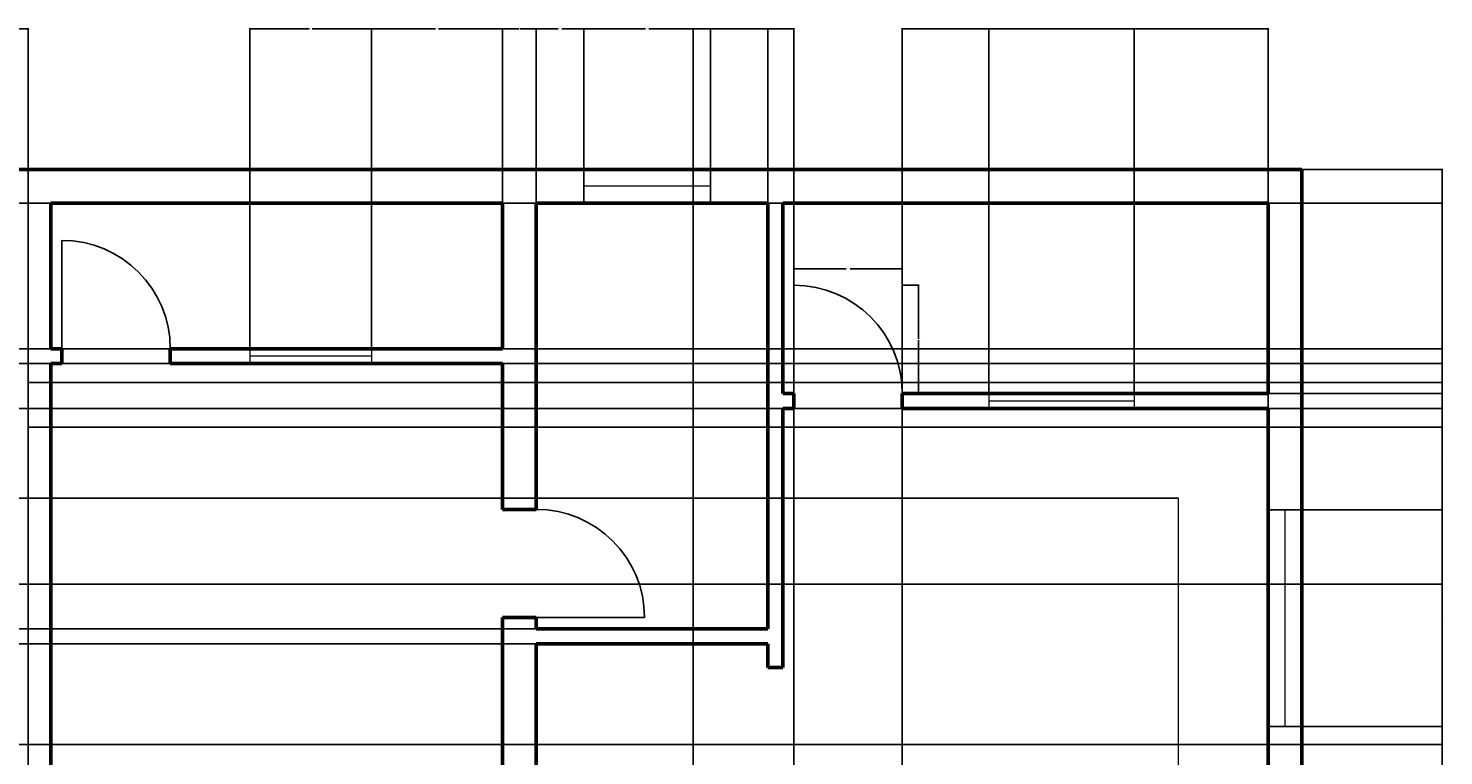
# Model space of a CAD drawing. Units: inches. Extents: x 2479 to 3284, y 2154 to 2936.
# Tile 8 of 8: x 2905 to 3284, y 2741 to 2936. Entities that reach past the tile are written whole.
import ezdxf

# ---------------------------------------------------------------- set-up
doc = ezdxf.new("R2010")
doc.units = ezdxf.units.IN
for name, color, linetype, lineweight in [('A-ANNO-DIMS', 2, 'Continuous', 18), ('A-DOOR', 3, 'Continuous', 25), ('A-FLOR-CASE', 8, 'Continuous', 18), ('A-GLAZ', 4, 'Continuous', 18), ('A-WALL', 7, 'Continuous', 50)]:
    doc.layers.add(name, color=color, linetype=linetype, lineweight=lineweight)
doc.styles.get("Standard").update_dxf_attribs({"font": 'arial.ttf'})
doc.dimstyles.get("Standard").update_dxf_attribs({"dimtxt": 0.18, "dimasz": 0.18, "dimexe": 0.18, "dimexo": 0.0625, "dimgap": 0.09, "dimtad": 0, "dimtih": 1, "dimtoh": 1, "dimdec": 4, "dimzin": 0, "dimdsep": 46, "dimtxsty": 'Standard', "dimcen": 0.09, "dimadec": 0, "dimazin": 0, "dimtfac": 1, "dimtdec": 4, "dimtofl": 0, "dimtmove": 0, "dimatfit": 3, "dimfxl": 1, "dimtolj": 1, "dimtzin": 0, "dimarcsym": 0})

# ---------------------------------------------------------------- blocks, each defined once
blk = doc.blocks.new('DOOR-SWING-29IN')
blk.add_line((29, 0), (0, 0))
blk.add_arc((29, 0), 29, 90, 180)
blk = doc.blocks.new('*D3')
at = {"layer": 'A-ANNO-DIMS', "color": 0, "lineweight": -2, "transparency": 16777216}
for p, q in [((3139.27, 2866.74), (3143.74, 2866.74)), ((3143.56, 2866.56), (3143.56, 2852.42)), ((3143.56, 2837.92), (3143.56, 2852.06)), ((3139.27, 2837.74), (3143.74, 2837.74))]:
    blk.add_line(p, q, dxfattribs=at)
at = {"layer": 'A-ANNO-DIMS', "color": 0, "transparency": 16777216}
for points in [[(3143.53, 2866.56), (3143.59, 2866.56), (3143.56, 2866.74)], [(3143.53, 2837.92), (3143.59, 2837.92), (3143.56, 2837.74)]]:
    blk.add_solid(points, dxfattribs=at)
at = {"layer": 'Defpoints', "color": 0, "transparency": 16777216}
for p in [(3139.21, 2866.74), (3139.21, 2837.74), (3143.56, 2837.74)]:
    blk.add_point(p, dxfattribs=at)
at = {"layer": 'A-ANNO-DIMS', "color": 0, "transparency": 16777216, "insert": (3143.56, 2852.24), "char_height": 0.18, "attachment_point": 5}
blk.add_mtext('\\A1;DOOR 29 TYP.', dxfattribs=at)
blk = doc.blocks.new('*D4')
at = {"layer": 'A-ANNO-DIMS', "color": 0, "lineweight": -2, "transparency": 16777216}
for p, q in [((3110.21, 2866.8), (3110.21, 2871.27)), ((3110.39, 2871.09), (3124.18, 2871.09)), ((3139.03, 2871.09), (3125.24, 2871.09)), ((3139.21, 2866.8), (3139.21, 2871.27))]:
    blk.add_line(p, q, dxfattribs=at)
at = {"layer": 'A-ANNO-DIMS', "color": 0, "transparency": 16777216}
for points in [[(3110.39, 2871.12), (3110.39, 2871.06), (3110.21, 2871.09)], [(3139.03, 2871.12), (3139.03, 2871.06), (3139.21, 2871.09)]]:
    blk.add_solid(points, dxfattribs=at)
at = {"layer": 'Defpoints', "color": 0, "transparency": 16777216}
for p in [(3139.21, 2871.09), (3110.21, 2866.74), (3139.21, 2866.74)]:
    blk.add_point(p, dxfattribs=at)
at = {"layer": 'A-ANNO-DIMS', "color": 0, "transparency": 16777216, "insert": (3124.71, 2871.09), "char_height": 0.18, "attachment_point": 5}
blk.add_mtext('\\A1;29 TYP.', dxfattribs=at)
blk = doc.blocks.new('*D9')
at = {"layer": 'A-ANNO-DIMS', "color": 0, "lineweight": -2, "transparency": 16777216}
for p, q in [((2517.21, 2897.8), (2517.21, 2935.52)), ((2517.39, 2935.34), (2710.92, 2935.34)), ((2905.03, 2935.34), (2711.5, 2935.34)), ((2905.21, 2888.8), (2905.21, 2935.52))]:
    blk.add_line(p, q, dxfattribs=at)
at = {"layer": 'A-ANNO-DIMS', "color": 0, "transparency": 16777216}
for points in [[(2517.39, 2935.37), (2517.39, 2935.31), (2517.21, 2935.34)], [(2905.03, 2935.37), (2905.03, 2935.31), (2905.21, 2935.34)]]:
    blk.add_solid(points, dxfattribs=at)
at = {"layer": 'Defpoints', "color": 0, "transparency": 16777216}
for p in [(2905.21, 2935.34), (2517.21, 2897.74), (2905.21, 2888.74)]:
    blk.add_point(p, dxfattribs=at)
at = {"layer": 'A-ANNO-DIMS', "color": 0, "transparency": 16777216, "insert": (2711.21, 2935.34), "char_height": 0.18, "attachment_point": 5}
blk.add_mtext('\\A1;388', dxfattribs=at)
blk = doc.blocks.new('*D10')
at = {"layer": 'A-ANNO-DIMS', "color": 0, "lineweight": -2, "transparency": 16777216}
for p, q in [((3246.27, 2897.74), (3283.99, 2897.74)), ((3283.81, 2897.56), (3283.81, 2715.92)), ((3283.81, 2533.92), (3283.81, 2715.56)), ((3237.27, 2533.74), (3283.99, 2533.74))]:
    blk.add_line(p, q, dxfattribs=at)
at = {"layer": 'A-ANNO-DIMS', "color": 0, "transparency": 16777216}
for points in [[(3283.78, 2897.56), (3283.84, 2897.56), (3283.81, 2897.74)], [(3283.78, 2533.92), (3283.84, 2533.92), (3283.81, 2533.74)]]:
    blk.add_solid(points, dxfattribs=at)
at = {"layer": 'Defpoints', "color": 0, "transparency": 16777216}
for p in [(3246.21, 2897.74), (3283.81, 2897.74), (3237.21, 2533.74)]:
    blk.add_point(p, dxfattribs=at)
at = {"layer": 'A-ANNO-DIMS', "color": 0, "transparency": 16777216, "insert": (3283.81, 2715.74), "char_height": 0.18, "attachment_point": 5}
blk.add_mtext('\\A1;364', dxfattribs=at)
blk = doc.blocks.new('*D11')
at = {"layer": 'A-ANNO-DIMS', "color": 0, "lineweight": -2, "transparency": 16777216}
for p, q in [((2845.21, 2542.8), (2845.21, 2935.52)), ((2845.39, 2935.34), (2874.99, 2935.34)), ((2905.03, 2935.34), (2875.43, 2935.34)), ((2905.21, 2542.8), (2905.21, 2935.52))]:
    blk.add_line(p, q, dxfattribs=at)
at = {"layer": 'A-ANNO-DIMS', "color": 0, "transparency": 16777216}
for points in [[(2845.39, 2935.37), (2845.39, 2935.31), (2845.21, 2935.34)], [(2905.03, 2935.37), (2905.03, 2935.31), (2905.21, 2935.34)]]:
    blk.add_solid(points, dxfattribs=at)
at = {"layer": 'Defpoints', "color": 0, "transparency": 16777216}
for p in [(2905.21, 2935.34), (2845.21, 2542.74), (2905.21, 2542.74)]:
    blk.add_point(p, dxfattribs=at)
at = {"layer": 'A-ANNO-DIMS', "color": 0, "transparency": 16777216, "insert": (2875.21, 2935.34), "char_height": 0.18, "attachment_point": 5}
blk.add_mtext('\\A1;60', dxfattribs=at)
blk = doc.blocks.new('*D32')
at = {"layer": 'A-ANNO-DIMS', "color": 0, "lineweight": -2, "transparency": 16777216}
for p, q in [((2905.27, 2840.74), (3283.99, 2840.74)), ((3283.81, 2840.56), (3283.81, 2834.92)), ((3283.81, 2828.92), (3283.81, 2834.56)), ((2905.27, 2828.74), (3283.99, 2828.74))]:
    blk.add_line(p, q, dxfattribs=at)
at = {"layer": 'A-ANNO-DIMS', "color": 0, "transparency": 16777216}
for points in [[(3283.78, 2840.56), (3283.84, 2840.56), (3283.81, 2840.74)], [(3283.78, 2828.92), (3283.84, 2828.92), (3283.81, 2828.74)]]:
    blk.add_solid(points, dxfattribs=at)
at = {"layer": 'Defpoints', "color": 0, "transparency": 16777216}
for p in [(2905.21, 2840.74), (3283.81, 2840.74), (2905.21, 2828.74)]:
    blk.add_point(p, dxfattribs=at)
at = {"layer": 'A-ANNO-DIMS', "color": 0, "transparency": 16777216, "insert": (3283.81, 2834.74), "char_height": 0.18, "attachment_point": 5}
blk.add_mtext('\\A1;12', dxfattribs=at)
blk = doc.blocks.new('*D34')
at = {"layer": 'A-ANNO-DIMS', "color": 0, "lineweight": -2, "transparency": 16777216}
for p, q in [((2856.82, 2897.74), (3283.99, 2897.74)), ((3283.81, 2897.56), (3283.81, 2893.42)), ((3283.81, 2888.92), (3283.81, 2893.06)), ((2856.82, 2888.74), (3283.99, 2888.74))]:
    blk.add_line(p, q, dxfattribs=at)
at = {"layer": 'A-ANNO-DIMS', "color": 0, "transparency": 16777216}
for points in [[(3283.78, 2897.56), (3283.84, 2897.56), (3283.81, 2897.74)], [(3283.78, 2888.92), (3283.84, 2888.92), (3283.81, 2888.74)]]:
    blk.add_solid(points, dxfattribs=at)
at = {"layer": 'Defpoints', "color": 0, "transparency": 16777216}
for p in [(2856.76, 2897.74), (3283.81, 2897.74), (2856.76, 2888.74)]:
    blk.add_point(p, dxfattribs=at)
at = {"layer": 'A-ANNO-DIMS', "color": 0, "transparency": 16777216, "insert": (3283.81, 2893.24), "char_height": 0.18, "attachment_point": 5}
blk.add_mtext('\\A1;9', dxfattribs=at)
blk = doc.blocks.new('*D58')
at = {"layer": 'A-ANNO-DIMS', "color": 0, "lineweight": -2, "transparency": 16777216}
for p, q in [((2718.27, 2888.74), (3283.99, 2888.74)), ((3283.81, 2888.56), (3283.81, 2869.42)), ((3283.81, 2849.92), (3283.81, 2869.06)), ((2718.27, 2849.74), (3283.99, 2849.74))]:
    blk.add_line(p, q, dxfattribs=at)
at = {"layer": 'A-ANNO-DIMS', "color": 0, "transparency": 16777216}
for points in [[(3283.78, 2888.56), (3283.84, 2888.56), (3283.81, 2888.74)], [(3283.78, 2849.92), (3283.84, 2849.92), (3283.81, 2849.74)]]:
    blk.add_solid(points, dxfattribs=at)
at = {"layer": 'Defpoints', "color": 0, "transparency": 16777216}
for p in [(2718.21, 2888.74), (3283.81, 2888.74), (2718.21, 2849.74)]:
    blk.add_point(p, dxfattribs=at)
at = {"layer": 'A-ANNO-DIMS', "color": 0, "transparency": 16777216, "insert": (3283.81, 2869.24), "char_height": 0.18, "attachment_point": 5}
blk.add_mtext('\\A1;39', dxfattribs=at)
blk = doc.blocks.new('*D59')
at = {"layer": 'A-ANNO-DIMS', "color": 0, "lineweight": -2, "transparency": 16777216}
for p, q in [((2839.27, 2845.74), (3283.99, 2845.74)), ((3283.81, 2845.56), (3283.81, 2816.42)), ((3283.81, 2786.92), (3283.81, 2816.06)), ((2712.27, 2786.74), (3283.99, 2786.74))]:
    blk.add_line(p, q, dxfattribs=at)
at = {"layer": 'A-ANNO-DIMS', "color": 0, "transparency": 16777216}
for points in [[(3283.78, 2845.56), (3283.84, 2845.56), (3283.81, 2845.74)], [(3283.78, 2786.92), (3283.84, 2786.92), (3283.81, 2786.74)]]:
    blk.add_solid(points, dxfattribs=at)
at = {"layer": 'Defpoints', "color": 0, "transparency": 16777216}
for p in [(2839.21, 2845.74), (3283.81, 2845.74), (2712.21, 2786.74)]:
    blk.add_point(p, dxfattribs=at)
at = {"layer": 'A-ANNO-DIMS', "color": 0, "transparency": 16777216, "insert": (3283.81, 2816.24), "char_height": 0.18, "attachment_point": 5}
blk.add_mtext('\\A1;59', dxfattribs=at)
blk = doc.blocks.new('*D60')
at = {"layer": 'A-ANNO-DIMS', "color": 0, "lineweight": -2, "transparency": 16777216}
for p, q in [((2712.27, 2786.74), (3283.99, 2786.74)), ((3283.81, 2786.56), (3283.81, 2765.42)), ((3283.81, 2743.92), (3283.81, 2765.06)), ((2839.27, 2743.74), (3283.99, 2743.74))]:
    blk.add_line(p, q, dxfattribs=at)
at = {"layer": 'A-ANNO-DIMS', "color": 0, "transparency": 16777216}
for points in [[(3283.78, 2786.56), (3283.84, 2786.56), (3283.81, 2786.74)], [(3283.78, 2743.92), (3283.84, 2743.92), (3283.81, 2743.74)]]:
    blk.add_solid(points, dxfattribs=at)
at = {"layer": 'Defpoints', "color": 0, "transparency": 16777216}
for p in [(2712.21, 2786.74), (3283.81, 2786.74), (2839.21, 2743.74)]:
    blk.add_point(p, dxfattribs=at)
at = {"layer": 'A-ANNO-DIMS', "color": 0, "transparency": 16777216, "insert": (3283.81, 2765.24), "char_height": 0.18, "attachment_point": 5}
blk.add_mtext('\\A1;43', dxfattribs=at)
blk = doc.blocks.new('*D66')
at = {"layer": 'A-ANNO-DIMS', "color": 0, "lineweight": -2, "transparency": 16777216}
for p, q in [((2964.49, 2849.8), (2964.49, 2935.52)), ((2964.67, 2935.34), (2980.39, 2935.34)), ((2996.9, 2935.34), (2981.18, 2935.34)), ((2997.08, 2849.8), (2997.08, 2935.52))]:
    blk.add_line(p, q, dxfattribs=at)
at = {"layer": 'A-ANNO-DIMS', "color": 0, "transparency": 16777216}
for points in [[(2964.67, 2935.37), (2964.67, 2935.31), (2964.49, 2935.34)], [(2996.9, 2935.37), (2996.9, 2935.31), (2997.08, 2935.34)]]:
    blk.add_solid(points, dxfattribs=at)
at = {"layer": 'Defpoints', "color": 0, "transparency": 16777216}
for p in [(2997.08, 2935.34), (2964.49, 2849.74), (2997.08, 2849.74)]:
    blk.add_point(p, dxfattribs=at)
at = {"layer": 'A-ANNO-DIMS', "color": 0, "transparency": 16777216, "insert": (2980.79, 2935.34), "char_height": 0.18, "attachment_point": 5}
blk.add_mtext('\\A1;32.59', dxfattribs=at)
blk = doc.blocks.new('*D67')
at = {"layer": 'A-ANNO-DIMS', "color": 0, "lineweight": -2, "transparency": 16777216}
for p, q in [((2997.08, 2849.8), (2997.08, 2935.52)), ((2997.26, 2935.34), (3014.25, 2935.34)), ((3032.03, 2935.34), (3015.04, 2935.34)), ((3032.21, 2849.8), (3032.21, 2935.52))]:
    blk.add_line(p, q, dxfattribs=at)
at = {"layer": 'A-ANNO-DIMS', "color": 0, "transparency": 16777216}
for points in [[(2997.26, 2935.37), (2997.26, 2935.31), (2997.08, 2935.34)], [(3032.03, 2935.37), (3032.03, 2935.31), (3032.21, 2935.34)]]:
    blk.add_solid(points, dxfattribs=at)
at = {"layer": 'Defpoints', "color": 0, "transparency": 16777216}
for p in [(3032.21, 2935.34), (2997.08, 2849.74), (3032.21, 2849.74)]:
    blk.add_point(p, dxfattribs=at)
at = {"layer": 'A-ANNO-DIMS', "color": 0, "transparency": 16777216, "insert": (3014.64, 2935.34), "char_height": 0.18, "attachment_point": 5}
blk.add_mtext('\\A1;35.13', dxfattribs=at)
blk = doc.blocks.new('*D68')
at = {"layer": 'A-ANNO-DIMS', "color": 0, "lineweight": -2, "transparency": 16777216}
for p, q in [((3032.21, 2888.8), (3032.21, 2935.52)), ((3032.39, 2935.34), (3036.56, 2935.34)), ((3041.03, 2935.34), (3036.86, 2935.34)), ((3041.21, 2888.8), (3041.21, 2935.52))]:
    blk.add_line(p, q, dxfattribs=at)
at = {"layer": 'A-ANNO-DIMS', "color": 0, "transparency": 16777216}
for points in [[(3032.39, 2935.37), (3032.39, 2935.31), (3032.21, 2935.34)], [(3041.03, 2935.37), (3041.03, 2935.31), (3041.21, 2935.34)]]:
    blk.add_solid(points, dxfattribs=at)
at = {"layer": 'Defpoints', "color": 0, "transparency": 16777216}
for p in [(3041.21, 2935.34), (3032.21, 2888.74), (3041.21, 2888.74)]:
    blk.add_point(p, dxfattribs=at)
at = {"layer": 'A-ANNO-DIMS', "color": 0, "transparency": 16777216, "insert": (3036.71, 2935.34), "char_height": 0.18, "attachment_point": 5}
blk.add_mtext('\\A1;9', dxfattribs=at)
blk = doc.blocks.new('*D69')
at = {"layer": 'A-ANNO-DIMS', "color": 0, "lineweight": -2, "transparency": 16777216}
for p, q in [((3041.21, 2888.8), (3041.21, 2935.52)), ((3041.39, 2935.34), (3047.12, 2935.34)), ((3053.76, 2935.34), (3048.03, 2935.34)), ((3053.94, 2888.8), (3053.94, 2935.52))]:
    blk.add_line(p, q, dxfattribs=at)
at = {"layer": 'A-ANNO-DIMS', "color": 0, "transparency": 16777216}
for points in [[(3041.39, 2935.37), (3041.39, 2935.31), (3041.21, 2935.34)], [(3053.76, 2935.37), (3053.76, 2935.31), (3053.94, 2935.34)]]:
    blk.add_solid(points, dxfattribs=at)
at = {"layer": 'Defpoints', "color": 0, "transparency": 16777216}
for p in [(3053.94, 2935.34), (3041.21, 2888.74), (3053.94, 2888.74)]:
    blk.add_point(p, dxfattribs=at)
at = {"layer": 'A-ANNO-DIMS', "color": 0, "transparency": 16777216, "insert": (3047.57, 2935.34), "char_height": 0.18, "attachment_point": 5}
blk.add_mtext('\\A1;12.727', dxfattribs=at)
blk = doc.blocks.new('*D70')
at = {"layer": 'A-ANNO-DIMS', "color": 0, "lineweight": -2, "transparency": 16777216}
for p, q in [((3053.94, 2888.8), (3053.94, 2935.52)), ((3054.12, 2935.34), (3070.42, 2935.34)), ((3087.66, 2935.34), (3071.35, 2935.34)), ((3087.84, 2888.8), (3087.84, 2935.52))]:
    blk.add_line(p, q, dxfattribs=at)
at = {"layer": 'A-ANNO-DIMS', "color": 0, "transparency": 16777216}
for points in [[(3054.12, 2935.37), (3054.12, 2935.31), (3053.94, 2935.34)], [(3087.66, 2935.37), (3087.66, 2935.31), (3087.84, 2935.34)]]:
    blk.add_solid(points, dxfattribs=at)
at = {"layer": 'Defpoints', "color": 0, "transparency": 16777216}
for p in [(3087.84, 2935.34), (3053.94, 2888.74), (3087.84, 2888.74)]:
    blk.add_point(p, dxfattribs=at)
at = {"layer": 'A-ANNO-DIMS', "color": 0, "transparency": 16777216, "insert": (3070.89, 2935.34), "char_height": 0.18, "attachment_point": 5}
blk.add_mtext('\\A1;33.905', dxfattribs=at)
blk = doc.blocks.new('*D71')
at = {"layer": 'A-ANNO-DIMS', "color": 0, "lineweight": -2, "transparency": 16777216}
for p, q in [((3087.84, 2888.8), (3087.84, 2935.52)), ((3088.02, 2935.34), (3095.07, 2935.34)), ((3103.03, 2935.34), (3095.98, 2935.34)), ((3103.21, 2888.8), (3103.21, 2935.52))]:
    blk.add_line(p, q, dxfattribs=at)
at = {"layer": 'A-ANNO-DIMS', "color": 0, "transparency": 16777216}
for points in [[(3088.02, 2935.37), (3088.02, 2935.31), (3087.84, 2935.34)], [(3103.03, 2935.37), (3103.03, 2935.31), (3103.21, 2935.34)]]:
    blk.add_solid(points, dxfattribs=at)
at = {"layer": 'Defpoints', "color": 0, "transparency": 16777216}
for p in [(3103.21, 2935.34), (3087.84, 2888.74), (3103.21, 2888.74)]:
    blk.add_point(p, dxfattribs=at)
at = {"layer": 'A-ANNO-DIMS', "color": 0, "transparency": 16777216, "insert": (3095.52, 2935.34), "char_height": 0.18, "attachment_point": 5}
blk.add_mtext('\\A1;15.368', dxfattribs=at)
blk = doc.blocks.new('*D72')
at = {"layer": 'A-ANNO-DIMS', "color": 0, "lineweight": -2, "transparency": 16777216}
for p, q in [((3162.36, 2837.8), (3162.36, 2935.52)), ((3162.54, 2935.34), (3181.36, 2935.34)), ((3201.1, 2935.34), (3182.28, 2935.34)), ((3201.28, 2837.8), (3201.28, 2935.52))]:
    blk.add_line(p, q, dxfattribs=at)
at = {"layer": 'A-ANNO-DIMS', "color": 0, "transparency": 16777216}
for points in [[(3162.54, 2935.37), (3162.54, 2935.31), (3162.36, 2935.34)], [(3201.1, 2935.37), (3201.1, 2935.31), (3201.28, 2935.34)]]:
    blk.add_solid(points, dxfattribs=at)
at = {"layer": 'Defpoints', "color": 0, "transparency": 16777216}
for p in [(3201.28, 2935.34), (3162.36, 2837.74), (3201.28, 2837.74)]:
    blk.add_point(p, dxfattribs=at)
at = {"layer": 'A-ANNO-DIMS', "color": 0, "transparency": 16777216, "insert": (3181.82, 2935.34), "char_height": 0.18, "attachment_point": 5}
blk.add_mtext('\\A1;38.914', dxfattribs=at)
blk = doc.blocks.new('*D73')
at = {"layer": 'A-ANNO-DIMS', "color": 0, "lineweight": -2, "transparency": 16777216}
for p, q in [((3201.28, 2837.8), (3201.28, 2935.52)), ((3201.46, 2935.34), (3218.85, 2935.34)), ((3237.03, 2935.34), (3219.64, 2935.34)), ((3237.21, 2837.8), (3237.21, 2935.52))]:
    blk.add_line(p, q, dxfattribs=at)
at = {"layer": 'A-ANNO-DIMS', "color": 0, "transparency": 16777216}
for points in [[(3201.46, 2935.37), (3201.46, 2935.31), (3201.28, 2935.34)], [(3237.03, 2935.37), (3237.03, 2935.31), (3237.21, 2935.34)]]:
    blk.add_solid(points, dxfattribs=at)
at = {"layer": 'Defpoints', "color": 0, "transparency": 16777216}
for p in [(3237.21, 2935.34), (3201.28, 2837.74), (3237.21, 2837.74)]:
    blk.add_point(p, dxfattribs=at)
at = {"layer": 'A-ANNO-DIMS', "color": 0, "transparency": 16777216, "insert": (3219.24, 2935.34), "char_height": 0.18, "attachment_point": 5}
blk.add_mtext('\\A1;35.93', dxfattribs=at)
blk = doc.blocks.new('*D80')
at = {"layer": 'A-ANNO-DIMS', "color": 0, "lineweight": -2, "transparency": 16777216}
for p, q in [((3237.27, 2748.61), (3283.99, 2748.61)), ((3283.81, 2748.43), (3283.81, 2734.36)), ((3283.81, 2719.92), (3283.81, 2733.99)), ((3237.27, 2719.74), (3283.99, 2719.74))]:
    blk.add_line(p, q, dxfattribs=at)
at = {"layer": 'A-ANNO-DIMS', "color": 0, "transparency": 16777216}
for points in [[(3283.78, 2748.43), (3283.84, 2748.43), (3283.81, 2748.61)], [(3283.78, 2719.92), (3283.84, 2719.92), (3283.81, 2719.74)]]:
    blk.add_solid(points, dxfattribs=at)
at = {"layer": 'Defpoints', "color": 0, "transparency": 16777216}
for p in [(3237.21, 2748.61), (3283.81, 2748.61), (3237.21, 2719.74)]:
    blk.add_point(p, dxfattribs=at)
at = {"layer": 'A-ANNO-DIMS', "color": 0, "transparency": 16777216, "insert": (3283.81, 2734.18), "char_height": 0.18, "attachment_point": 5}
blk.add_mtext('\\A1;28.874', dxfattribs=at)
blk = doc.blocks.new('*D81')
at = {"layer": 'A-ANNO-DIMS', "color": 0, "lineweight": -2, "transparency": 16777216}
for p, q in [((3237.27, 2806.65), (3283.99, 2806.65)), ((3283.81, 2806.47), (3283.81, 2777.82)), ((3283.81, 2748.79), (3283.81, 2777.45)), ((3237.27, 2748.61), (3283.99, 2748.61))]:
    blk.add_line(p, q, dxfattribs=at)
at = {"layer": 'A-ANNO-DIMS', "color": 0, "transparency": 16777216}
for points in [[(3283.78, 2806.47), (3283.84, 2806.47), (3283.81, 2806.65)], [(3283.78, 2748.79), (3283.84, 2748.79), (3283.81, 2748.61)]]:
    blk.add_solid(points, dxfattribs=at)
at = {"layer": 'Defpoints', "color": 0, "transparency": 16777216}
for p in [(3237.21, 2806.65), (3283.81, 2806.65), (3237.21, 2748.61)]:
    blk.add_point(p, dxfattribs=at)
at = {"layer": 'A-ANNO-DIMS', "color": 0, "transparency": 16777216, "insert": (3283.81, 2777.63), "char_height": 0.18, "attachment_point": 5}
blk.add_mtext('\\A1;58.04', dxfattribs=at)
blk = doc.blocks.new('*D82')
at = {"layer": 'A-ANNO-DIMS', "color": 0, "lineweight": -2, "transparency": 16777216}
for p, q in [((3237.27, 2833.74), (3283.99, 2833.74)), ((3283.81, 2833.56), (3283.81, 2820.38)), ((3283.81, 2806.83), (3283.81, 2820.02)), ((3237.27, 2806.65), (3283.99, 2806.65))]:
    blk.add_line(p, q, dxfattribs=at)
at = {"layer": 'A-ANNO-DIMS', "color": 0, "transparency": 16777216}
for points in [[(3283.78, 2833.56), (3283.84, 2833.56), (3283.81, 2833.74)], [(3283.78, 2806.83), (3283.84, 2806.83), (3283.81, 2806.65)]]:
    blk.add_solid(points, dxfattribs=at)
at = {"layer": 'Defpoints', "color": 0, "transparency": 16777216}
for p in [(3237.21, 2833.74), (3283.81, 2833.74), (3237.21, 2806.65)]:
    blk.add_point(p, dxfattribs=at)
at = {"layer": 'A-ANNO-DIMS', "color": 0, "transparency": 16777216, "insert": (3283.81, 2820.2), "char_height": 0.18, "attachment_point": 5}
blk.add_mtext('\\A1;27.085', dxfattribs=at)
blk = doc.blocks.new('*D83')
at = {"layer": 'A-ANNO-DIMS', "color": 0, "lineweight": -2, "transparency": 16777216}
for p, q in [((3237.27, 2888.74), (3283.99, 2888.74)), ((3283.81, 2888.56), (3283.81, 2863.42)), ((3283.81, 2837.92), (3283.81, 2863.06)), ((3237.27, 2837.74), (3283.99, 2837.74))]:
    blk.add_line(p, q, dxfattribs=at)
at = {"layer": 'A-ANNO-DIMS', "color": 0, "transparency": 16777216}
for points in [[(3283.78, 2888.56), (3283.84, 2888.56), (3283.81, 2888.74)], [(3283.78, 2837.92), (3283.84, 2837.92), (3283.81, 2837.74)]]:
    blk.add_solid(points, dxfattribs=at)
at = {"layer": 'Defpoints', "color": 0, "transparency": 16777216}
for p in [(3237.21, 2888.74), (3283.81, 2888.74), (3237.21, 2837.74)]:
    blk.add_point(p, dxfattribs=at)
at = {"layer": 'A-ANNO-DIMS', "color": 0, "transparency": 16777216, "insert": (3283.81, 2863.24), "char_height": 0.18, "attachment_point": 5}
blk.add_mtext('\\A1;51', dxfattribs=at)
blk = doc.blocks.new('*D84')
at = {"layer": 'A-ANNO-DIMS', "color": 0, "lineweight": -2, "transparency": 16777216}
for p, q in [((3032.15, 2888.74), (2479.43, 2888.74)), ((2479.61, 2888.56), (2479.61, 2869.42)), ((2479.61, 2849.92), (2479.61, 2869.06)), ((3032.15, 2849.74), (2479.43, 2849.74))]:
    blk.add_line(p, q, dxfattribs=at)
at = {"layer": 'A-ANNO-DIMS', "color": 0, "transparency": 16777216}
for points in [[(2479.58, 2888.56), (2479.64, 2888.56), (2479.61, 2888.74)], [(2479.58, 2849.92), (2479.64, 2849.92), (2479.61, 2849.74)]]:
    blk.add_solid(points, dxfattribs=at)
at = {"layer": 'Defpoints', "color": 0, "transparency": 16777216}
for p in [(2479.61, 2888.74), (3032.21, 2888.74), (3032.21, 2849.74)]:
    blk.add_point(p, dxfattribs=at)
at = {"layer": 'A-ANNO-DIMS', "color": 0, "transparency": 16777216, "insert": (2479.61, 2869.24), "char_height": 0.18, "attachment_point": 5}
blk.add_mtext('\\A1;39', dxfattribs=at)
blk = doc.blocks.new('*D85')
at = {"layer": 'A-ANNO-DIMS', "color": 0, "lineweight": -2, "transparency": 16777216}
for p, q in [((2911.15, 2845.74), (2479.43, 2845.74)), ((2479.61, 2845.56), (2479.61, 2810.42)), ((2479.61, 2774.92), (2479.61, 2810.06)), ((3041.15, 2774.74), (2479.43, 2774.74))]:
    blk.add_line(p, q, dxfattribs=at)
at = {"layer": 'A-ANNO-DIMS', "color": 0, "transparency": 16777216}
for points in [[(2479.58, 2845.56), (2479.64, 2845.56), (2479.61, 2845.74)], [(2479.58, 2774.92), (2479.64, 2774.92), (2479.61, 2774.74)]]:
    blk.add_solid(points, dxfattribs=at)
at = {"layer": 'Defpoints', "color": 0, "transparency": 16777216}
for p in [(2479.61, 2845.74), (2911.21, 2845.74), (3041.21, 2774.74)]:
    blk.add_point(p, dxfattribs=at)
at = {"layer": 'A-ANNO-DIMS', "color": 0, "transparency": 16777216, "insert": (2479.61, 2810.24), "char_height": 0.18, "attachment_point": 5}
blk.add_mtext('\\A1;71', dxfattribs=at)
blk = doc.blocks.new('*D86')
at = {"layer": 'A-ANNO-DIMS', "color": 0, "lineweight": -2, "transparency": 16777216}
for p, q in [((3041.15, 2770.74), (2479.43, 2770.74)), ((2479.61, 2770.56), (2479.61, 2715.42)), ((2479.61, 2659.92), (2479.61, 2715.06)), ((2911.15, 2659.74), (2479.43, 2659.74))]:
    blk.add_line(p, q, dxfattribs=at)
at = {"layer": 'A-ANNO-DIMS', "color": 0, "transparency": 16777216}
for points in [[(2479.58, 2770.56), (2479.64, 2770.56), (2479.61, 2770.74)], [(2479.58, 2659.92), (2479.64, 2659.92), (2479.61, 2659.74)]]:
    blk.add_solid(points, dxfattribs=at)
at = {"layer": 'Defpoints', "color": 0, "transparency": 16777216}
for p in [(2479.61, 2770.74), (3041.21, 2770.74), (2911.21, 2659.74)]:
    blk.add_point(p, dxfattribs=at)
at = {"layer": 'A-ANNO-DIMS', "color": 0, "transparency": 16777216, "insert": (2479.61, 2715.24), "char_height": 0.18, "attachment_point": 5}
blk.add_mtext('\\A1;111', dxfattribs=at)
blk = doc.blocks.new('*D89')
at = {"layer": 'A-ANNO-DIMS', "color": 0, "lineweight": -2, "transparency": 16777216}
for p, q in [((3139.15, 2833.74), (2479.43, 2833.74)), ((2479.61, 2833.56), (2479.61, 2821.92)), ((2479.61, 2809.92), (2479.61, 2821.56)), ((3213.15, 2809.74), (2479.43, 2809.74))]:
    blk.add_line(p, q, dxfattribs=at)
at = {"layer": 'A-ANNO-DIMS', "color": 0, "transparency": 16777216}
for points in [[(2479.58, 2833.56), (2479.64, 2833.56), (2479.61, 2833.74)], [(2479.58, 2809.92), (2479.64, 2809.92), (2479.61, 2809.74)]]:
    blk.add_solid(points, dxfattribs=at)
at = {"layer": 'Defpoints', "color": 0, "transparency": 16777216}
for p in [(2479.61, 2833.74), (3139.21, 2833.74), (3213.21, 2809.74)]:
    blk.add_point(p, dxfattribs=at)
at = {"layer": 'A-ANNO-DIMS', "color": 0, "transparency": 16777216, "insert": (2479.61, 2821.74), "char_height": 0.18, "attachment_point": 5}
blk.add_mtext('\\A1;24', dxfattribs=at)
blk = doc.blocks.new('*D131')
at = {"layer": 'A-ANNO-DIMS', "color": 0, "lineweight": -2, "transparency": 16777216}
for p, q in [((3083.21, 2407.8), (3083.21, 2935.52)), ((3083.39, 2935.34), (3096.49, 2935.34)), ((3110.03, 2935.34), (3096.93, 2935.34)), ((3110.21, 2407.8), (3110.21, 2935.52))]:
    blk.add_line(p, q, dxfattribs=at)
at = {"layer": 'A-ANNO-DIMS', "color": 0, "transparency": 16777216}
for points in [[(3083.39, 2935.37), (3083.39, 2935.31), (3083.21, 2935.34)], [(3110.03, 2935.37), (3110.03, 2935.31), (3110.21, 2935.34)]]:
    blk.add_solid(points, dxfattribs=at)
at = {"layer": 'Defpoints', "color": 0, "transparency": 16777216}
for p in [(3110.21, 2935.34), (3083.21, 2407.74), (3110.21, 2407.74)]:
    blk.add_point(p, dxfattribs=at)
at = {"layer": 'A-ANNO-DIMS', "color": 0, "transparency": 16777216, "insert": (3096.71, 2935.34), "char_height": 0.18, "attachment_point": 5}
blk.add_mtext('\\A1;27', dxfattribs=at)
blk = doc.blocks.new('*D132')
at = {"layer": 'A-ANNO-DIMS', "color": 0, "lineweight": -2, "transparency": 16777216}
for p, q in [((3139.21, 2407.8), (3139.21, 2935.52)), ((3139.39, 2935.34), (3187.99, 2935.34)), ((3237.03, 2935.34), (3188.43, 2935.34)), ((3237.21, 2407.8), (3237.21, 2935.52))]:
    blk.add_line(p, q, dxfattribs=at)
at = {"layer": 'A-ANNO-DIMS', "color": 0, "transparency": 16777216}
for points in [[(3139.39, 2935.37), (3139.39, 2935.31), (3139.21, 2935.34)], [(3237.03, 2935.37), (3237.03, 2935.31), (3237.21, 2935.34)]]:
    blk.add_solid(points, dxfattribs=at)
at = {"layer": 'Defpoints', "color": 0, "transparency": 16777216}
for p in [(3237.21, 2935.34), (3139.21, 2407.74), (3237.21, 2407.74)]:
    blk.add_point(p, dxfattribs=at)
at = {"layer": 'A-ANNO-DIMS', "color": 0, "transparency": 16777216, "insert": (3188.21, 2935.34), "char_height": 0.18, "attachment_point": 5}
blk.add_mtext('\\A1;98', dxfattribs=at)

msp = doc.modelspace()

# ---------------------------------------------------------------- linework, layer by layer
at = {"layer": 'A-FLOR-CASE'}
for p, q in [((3139.2088, 2809.7397), (3139.2088, 2833.7397)), ((3213.2088, 2809.7397), (3139.2088, 2809.7397)), ((3213.2088, 2719.7397), (3213.2088, 2809.7397))]:
    msp.add_line(p, q, dxfattribs=at)
at = {"layer": 'A-GLAZ'}
for p, q in [((3053.9361, 2888.7397), (3053.9361, 2897.7397)), ((3087.8411, 2888.7397), (3087.8411, 2897.7397)), ((3087.8411, 2893.2397), (3053.9361, 2893.2397)), ((2964.4898, 2849.7397), (2964.4898, 2845.7397)), ((2997.0803, 2847.7397), (2964.4898, 2847.7397)), ((2997.0803, 2849.7397), (2997.0803, 2845.7397)), ((3162.362, 2837.7397), (3162.362, 2833.7397)), ((3201.2764, 2835.7397), (3162.362, 2835.7397)), ((3201.2764, 2837.7397), (3201.2764, 2833.7397)), ((3237.2088, 2806.6546), (3246.2088, 2806.6546)), ((3241.7088, 2748.6135), (3241.7088, 2806.6546)), ((3237.2088, 2748.6135), (3246.2088, 2748.6135))]:
    msp.add_line(p, q, dxfattribs=at)
at = {"layer": 'A-WALL'}
for p, q in [((3246.2088, 2897.7397), (2517.2088, 2897.7397)), ((3246.2088, 2191.7397), (3246.2088, 2897.7397)), ((2911.2088, 2888.7397), (2911.2088, 2849.7397)), ((3032.2088, 2888.7397), (2911.2088, 2888.7397)), ((3032.2088, 2888.7397), (3032.2088, 2849.7397)), ((3041.2088, 2888.7397), (3041.2088, 2806.7397)), ((3103.2088, 2888.7397), (3041.2088, 2888.7397)), ((3103.2088, 2888.7397), (3103.2088, 2774.7397)), ((3237.2088, 2888.7397), (3107.2088, 2888.7397)), ((3107.2088, 2888.7397), (3107.2088, 2837.7397)), ((3237.2088, 2837.7397), (3237.2088, 2888.7397)), ((2914.2088, 2849.7397), (2911.2088, 2849.7397)), ((2914.2088, 2849.7397), (2914.2088, 2845.7397)), ((3032.2088, 2849.7397), (2943.2088, 2849.7397)), ((2943.2088, 2849.7397), (2943.2088, 2845.7397)), ((2911.2088, 2845.7397), (2911.2088, 2659.7397)), ((2914.2088, 2845.7397), (2911.2088, 2845.7397)), ((3032.2088, 2845.7397), (2943.2088, 2845.7397)), ((3032.2088, 2845.7397), (3032.2088, 2806.7397)), ((3110.2088, 2837.7397), (3107.2088, 2837.7397)), ((3110.2088, 2837.7397), (3110.2088, 2833.7397)), ((3237.2088, 2837.7397), (3139.2088, 2837.7397)), ((3139.2088, 2837.7397), (3139.2088, 2833.7397)), ((3110.2088, 2833.7397), (3107.2088, 2833.7397)), ((3107.2088, 2833.7397), (3107.2088, 2764.3559)), ((3237.2088, 2833.7397), (3139.2088, 2833.7397)), ((3237.2088, 2719.7397), (3237.2088, 2833.7397)), ((3041.2088, 2806.7397), (3032.2088, 2806.7397)), ((3041.2088, 2777.7397), (3032.2088, 2777.7397)), ((3032.2088, 2777.7397), (3032.2088, 2698.7397)), ((3041.2088, 2777.7397), (3041.2088, 2774.7397)), ((3103.2088, 2774.7397), (3041.2088, 2774.7397)), ((3103.2088, 2770.7397), (3041.2088, 2770.7397)), ((3041.2088, 2770.7397), (3041.2088, 2698.7397)), ((3103.2088, 2770.7397), (3103.2088, 2764.3559)), ((3107.2088, 2764.3559), (3103.2088, 2764.3559))]:
    msp.add_line(p, q, dxfattribs=at)

# ---------------------------------------------------------------- block references
at = {"layer": 'A-DOOR', "rotation": 270}
for p in [(2914.2088, 2878.7397), (3110.2088, 2866.7397)]:
    msp.add_blockref('DOOR-SWING-29IN', p, dxfattribs=at)
at = {"layer": 'A-DOOR', "extrusion": (0, 0, -1), "zscale": -1}
msp.add_blockref('DOOR-SWING-29IN', (-3070.2088, 2777.7397), dxfattribs=at)

# ---------------------------------------------------------------- dimensions: what is measured, and where the dimension line sits
at = {"layer": 'A-ANNO-DIMS'}
for base, p1, p2, override, picture, middle in [((2905.2088, 2935.3397), (2517.2088, 2897.7397), (2905.2088, 2888.7397), {"dimdec": 0, "dimlfac": 1, "dimrnd": 0, "dimzin": 0, "dimdsep": 46, "dimlunit": 2}, '*D9', (2711.2088, 2935.3397)), ((2905.2088, 2935.3397), (2845.2088, 2542.7397), (2905.2088, 2542.7397), {"dimdec": 0, "dimlfac": 1, "dimrnd": 0, "dimzin": 0, "dimdsep": 46, "dimlunit": 2}, '*D11', (2875.2088, 2935.3397)), ((2997.0803, 2935.3397), (2964.4898, 2849.7397), (2997.0803, 2849.7397), {"dimdec": 2, "dimlfac": 1, "dimrnd": 0, "dimzin": 0, "dimdsep": 46, "dimlunit": 2}, '*D66', (2980.785, 2935.3397)), ((3032.2088, 2935.3397), (2997.0803, 2849.7397), (3032.2088, 2849.7397), {"dimdec": 2, "dimlfac": 1, "dimrnd": 0, "dimzin": 0, "dimdsep": 46, "dimlunit": 2}, '*D67', (3014.6446, 2935.3397)), ((3041.2088, 2935.3397), (3032.2088, 2888.7397), (3041.2088, 2888.7397), {"dimdec": 0, "dimlfac": 1, "dimrnd": 0, "dimzin": 0, "dimdsep": 46, "dimlunit": 2}, '*D68', (3036.7088, 2935.3397)), ((3053.9361, 2935.3397), (3041.2088, 2888.7397), (3053.9361, 2888.7397), {"dimdec": 3, "dimlfac": 1, "dimrnd": 0, "dimzin": 0, "dimdsep": 46, "dimlunit": 2}, '*D69', (3047.5725, 2935.3397)), ((3087.8411, 2935.3397), (3053.9361, 2888.7397), (3087.8411, 2888.7397), {"dimdec": 3, "dimlfac": 1, "dimrnd": 0, "dimzin": 0, "dimdsep": 46, "dimlunit": 2}, '*D70', (3070.8886, 2935.3397)), ((3110.2088, 2935.3397), (3083.2088, 2407.7397), (3110.2088, 2407.7397), {"dimdec": 0, "dimlfac": 1, "dimrnd": 0, "dimzin": 0, "dimdsep": 46, "dimlunit": 2}, '*D131', (3096.7088, 2935.3397)), ((3103.2088, 2935.3397), (3087.8411, 2888.7397), (3103.2088, 2888.7397), {"dimdec": 3, "dimlfac": 1, "dimrnd": 0, "dimzin": 0, "dimdsep": 46, "dimlunit": 2}, '*D71', (3095.5249, 2935.3397)), ((3237.2088, 2935.3397), (3139.2088, 2407.7397), (3237.2088, 2407.7397), {"dimdec": 0, "dimlfac": 1, "dimrnd": 0, "dimzin": 0, "dimdsep": 46, "dimlunit": 2}, '*D132', (3188.2088, 2935.3397)), ((3201.2764, 2935.3397), (3162.362, 2837.7397), (3201.2764, 2837.7397), {"dimdec": 3, "dimlfac": 1, "dimrnd": 0, "dimzin": 0, "dimdsep": 46, "dimlunit": 2}, '*D72', (3181.8192, 2935.3397)), ((3237.2088, 2935.3397), (3201.2764, 2837.7397), (3237.2088, 2837.7397), {"dimdec": 2, "dimlfac": 1, "dimrnd": 0, "dimzin": 0, "dimdsep": 46, "dimlunit": 2}, '*D73', (3219.2426, 2935.3397))]:
    dim = msp.add_linear_dim(base=base, p1=p1, p2=p2, dimstyle='Standard', override=override, dxfattribs=at)
    dim.commit()
    dim.dimension.update_dxf_attribs({"geometry": picture, "text_midpoint": middle})
for base, p1, p2, override, picture, middle in [((3283.8088, 2897.7397), (2856.7618, 2888.7397), (2856.7618, 2897.7397), {"dimdec": 0, "dimlfac": 1, "dimrnd": 0, "dimzin": 0, "dimdsep": 46, "dimlunit": 2}, '*D34', (3283.8088, 2893.2397)), ((3283.8088, 2897.7397), (3237.2088, 2533.7397), (3246.2088, 2897.7397), {"dimdec": 0, "dimlfac": 1, "dimrnd": 0, "dimzin": 0, "dimdsep": 46, "dimlunit": 2}, '*D10', (3283.8088, 2715.7397)), ((2479.6088, 2888.7397), (3032.2088, 2849.7397), (3032.2088, 2888.7397), {"dimdec": 0, "dimlfac": 1, "dimrnd": 0, "dimzin": 0, "dimdsep": 46, "dimlunit": 2}, '*D84', (2479.6088, 2869.2397)), ((3283.8088, 2888.7397), (2718.2088, 2849.7397), (2718.2088, 2888.7397), {"dimdec": 0, "dimlfac": 1, "dimrnd": 0, "dimzin": 0, "dimdsep": 46, "dimlunit": 2}, '*D58', (3283.8088, 2869.2397)), ((3283.8088, 2888.7397), (3237.2088, 2837.7397), (3237.2088, 2888.7397), {"dimdec": 0, "dimlfac": 1, "dimrnd": 0, "dimzin": 0, "dimdsep": 46, "dimlunit": 2}, '*D83', (3283.8088, 2863.2397)), ((2479.6088, 2845.7397), (3041.2088, 2774.7397), (2911.2088, 2845.7397), {"dimdec": 0, "dimlfac": 1, "dimrnd": 0, "dimzin": 0, "dimdsep": 46, "dimlunit": 2}, '*D85', (2479.6088, 2810.2397)), ((3283.8088, 2845.7397), (2712.2088, 2786.7397), (2839.2088, 2845.7397), {"dimdec": 0, "dimlfac": 1, "dimrnd": 0, "dimzin": 0, "dimdsep": 46, "dimlunit": 2}, '*D59', (3283.8088, 2816.2397)), ((3283.8088, 2840.7397), (2905.2088, 2828.7397), (2905.2088, 2840.7397), {"dimdec": 0, "dimlfac": 1, "dimrnd": 0, "dimzin": 0, "dimdsep": 46, "dimlunit": 2}, '*D32', (3283.8088, 2834.7397)), ((2479.6088, 2833.7397), (3213.2088, 2809.7397), (3139.2088, 2833.7397), {"dimdec": 0, "dimlfac": 1, "dimrnd": 0, "dimzin": 0, "dimdsep": 46, "dimlunit": 2}, '*D89', (2479.6088, 2821.7397)), ((3283.8088, 2833.7397), (3237.2088, 2806.6546), (3237.2088, 2833.7397), {"dimdec": 3, "dimlfac": 1, "dimrnd": 0, "dimzin": 0, "dimdsep": 46, "dimlunit": 2}, '*D82', (3283.8088, 2820.1972)), ((3283.8088, 2806.6546), (3237.2088, 2748.6135), (3237.2088, 2806.6546), {"dimdec": 2, "dimlfac": 1, "dimrnd": 0, "dimzin": 0, "dimdsep": 46, "dimlunit": 2}, '*D81', (3283.8088, 2777.634)), ((3283.8088, 2786.7397), (2839.2088, 2743.7397), (2712.2088, 2786.7397), {"dimdec": 0, "dimlfac": 1, "dimrnd": 0, "dimzin": 0, "dimdsep": 46, "dimlunit": 2}, '*D60', (3283.8088, 2765.2397)), ((2479.6088, 2770.7397), (2911.2088, 2659.7397), (3041.2088, 2770.7397), {"dimdec": 0, "dimlfac": 1, "dimrnd": 0, "dimzin": 0, "dimdsep": 46, "dimlunit": 2}, '*D86', (2479.6088, 2715.2397)), ((3283.8088, 2748.6135), (3237.2088, 2719.7397), (3237.2088, 2748.6135), {"dimdec": 3, "dimlfac": 1, "dimrnd": 0, "dimzin": 0, "dimdsep": 46, "dimlunit": 2}, '*D80', (3283.8088, 2734.1766))]:
    dim = msp.add_linear_dim(base=base, p1=p1, p2=p2, angle=90, dimstyle='Standard', override=override, dxfattribs=at)
    dim.commit()
    dim.dimension.update_dxf_attribs({"geometry": picture, "text_midpoint": middle})
dim = msp.add_linear_dim(base=(3139.2088, 2871.0897), p1=(3110.2088, 2866.7397), p2=(3139.2088, 2866.7397), text='<> TYP.', dimstyle='Standard', override={"dimdec": 0, "dimlfac": 1, "dimrnd": 0, "dimzin": 0, "dimdsep": 46, "dimlunit": 2}, dxfattribs=at)
dim.commit()
dim.dimension.update_dxf_attribs({"geometry": '*D4', "text_midpoint": (3124.7088, 2871.0897)})
dim = msp.add_linear_dim(base=(3143.5588, 2837.7397), p1=(3139.2088, 2866.7397), p2=(3139.2088, 2837.7397), angle=270, text='DOOR <> TYP.', dimstyle='Standard', override={"dimdec": 0, "dimlfac": 1, "dimrnd": 0, "dimzin": 0, "dimdsep": 46, "dimlunit": 2}, dxfattribs=at)
dim.commit()
dim.dimension.update_dxf_attribs({"geometry": '*D3', "text_midpoint": (3143.5588, 2852.2397)})

doc.saveas('drawing.dxf')
